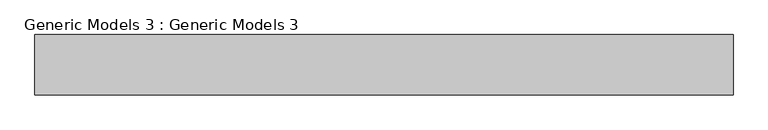
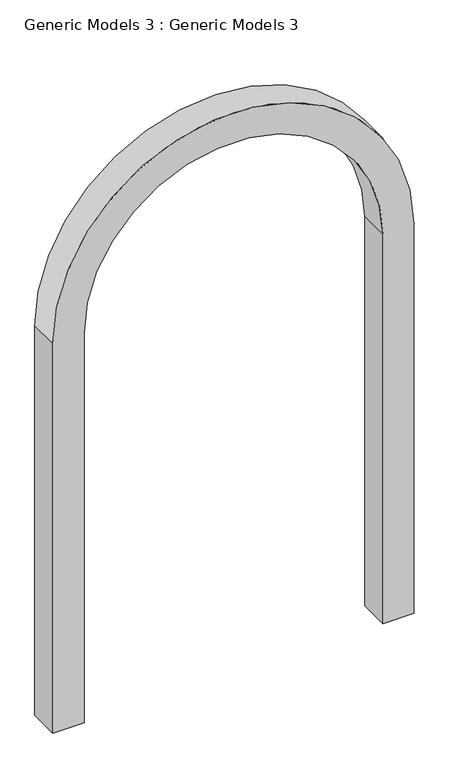
"""IFC4 building model written with IfcOpenShell, lengths in millimetres: proxy geometry, Generic Models 3 : Generic Models 3."""

from ifc_helpers import new_model, si_unit, point, frame, frame_2d, origin, place, context, project, spatial, polyline, circle_curve, trimmed, segment, composite_curve, outline, extrude, source, transform, mapped, element, save


def generic_models_3_generic_models_3_7bb868d1(model_context):
    return source(origin(), model_context, "Body", "SweptSolid", [
        extrude(outline(composite_curve([segment(trimmed(circle_curve(frame_2d((5031.4, -4097.4482439)), 609.6), [point((5031.4, -4707.0482439))], [point((5031.4, -3487.8482439))], True, "CARTESIAN"), True, "CONTINUOUS"), segment(polyline([(5031.4, -3487.8482439), (3352.8, -3487.8482439), (3352.8, -3360.8482439), (5031.4, -3360.8482439)]), True, "CONTINUOUS"), segment(trimmed(circle_curve(frame_2d((5031.4, -4097.4482439)), 736.6), [point((5031.4, -3360.8482439))], [point((5031.4, -4834.0482439))], False, "CARTESIAN"), True, "CONTINUOUS"), segment(polyline([(5031.4, -4834.0482439), (3352.8, -4834.0482439), (3352.8, -4707.0482439), (5031.4, -4707.0482439)]), True, "CONTINUOUS")], self_intersect=False)), frame((0.0, -5849.5827462, 0.0), z_axis=(0.0, 1.0, 0.0), x_axis=(0.0, 0.0, 1.0)), (0.0, 0.0, 1.0), 127.0),
    ])


if __name__ == "__main__":
    model = new_model("IFC4")
    model_context = context("Model", 3, world=origin())
    ifc_project = project(units=[si_unit("LENGTHUNIT", "METRE", prefix="MILLI")], contexts=[model_context])
    site = spatial("IfcSite", under=ifc_project)
    building = spatial("IfcBuilding", under=site)
    placement = place(None, origin())
    generic_models_3_generic_models_3_shape = generic_models_3_generic_models_3_7bb868d1(model_context)
    element("IfcBuildingElementProxy", 1, Name="Generic Models 3 : Generic Models 3", ObjectType="Generic Models 3 : Generic Models 3", at=placement, inside=building, context=model_context, shape_type="MappedRepresentation", body=[
        mapped(generic_models_3_generic_models_3_shape, transform((0.0, 0.0, 0.0), x_axis=(1.0, 0.0, 0.0), y_axis=(0.0, 1.0, 0.0), z_axis=(0.0, 0.0, 1.0))),
    ])
    save(model, "model.ifc")

# Revit data of these elements
# Element 1 (IfcBuildingElementProxy, "Generic Models 3 : Generic Models 3")
#   Materials on its faces: "BLACK"
# Materials
#   "BLACK": class "Generic", colour RGB 120 120 120, transparency 0, Cost = 0
